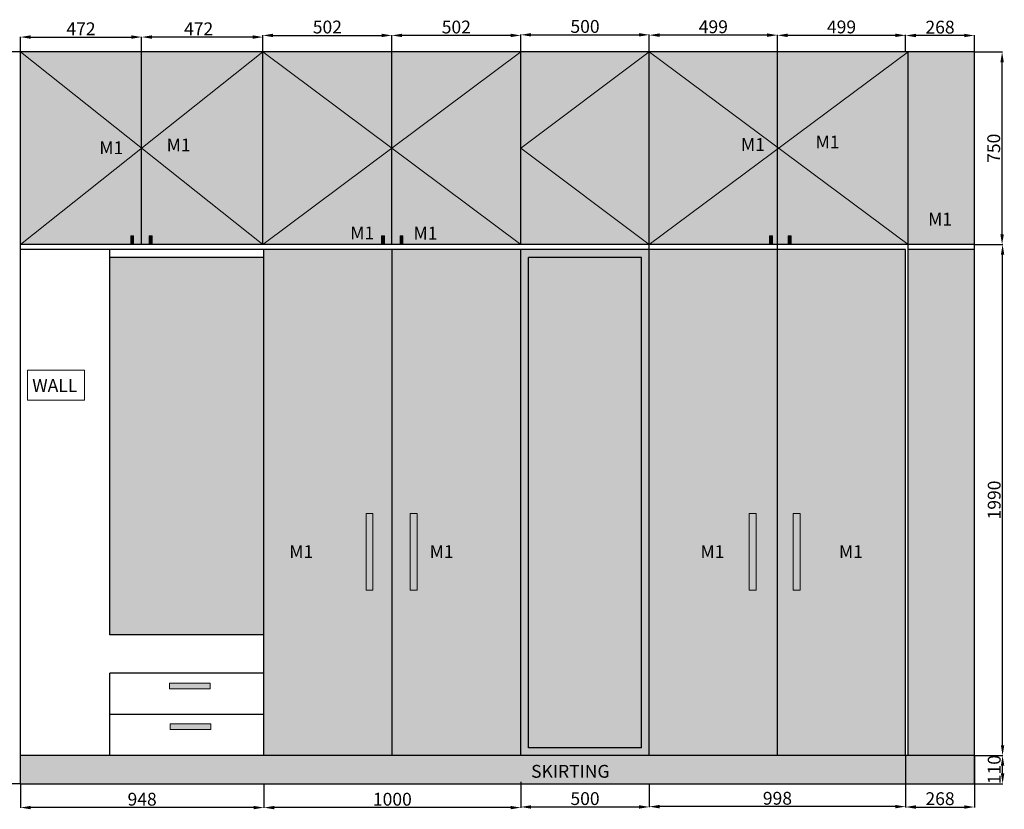
# Model space of a CAD drawing. Units: millimetres. Extents: x 46070 to 59439, y 6883 to 14761.
# Tile 2 of 5: x 49997 to 53830, y 6883 to 9959. Entities that reach past the tile are written whole.
import ezdxf

# ---------------------------------------------------------------- set-up
doc = ezdxf.new("R2010")
doc.units = ezdxf.units.MM
for name, color, linetype, lineweight in [('A-ANNO-DIMS', 2, 'Continuous', 18), ('A-ANNO-TEXT', 7, 'Continuous', 18), ('A-ELEV', 7, 'Continuous', 25), ('A-ELEV-OPEN', 1, 'Continuous', 13), ('A-ELEV-PATT', 8, 'Continuous', 13), ('A-FURN-HDWR', 4, 'Continuous', 18)]:
    doc.layers.add(name, color=color, linetype=linetype, lineweight=lineweight)
doc.styles.get("Standard").update_dxf_attribs({"font": 'arial.ttf'})
doc.dimstyles.new('ISO-25', dxfattribs={"dimtxt": 50, "dimasz": 40, "dimexe": 1.25, "dimexo": 0.625, "dimtad": 1, "dimtxsty": 'Standard', "dimcen": 2.5, "dimadec": 0, "dimazin": 0, "dimtfac": 1, "dimtmove": 0, "dimatfit": 3, "dimfxl": 1, "dimarcsym": 0})

# ---------------------------------------------------------------- blocks, each defined once
blk = doc.blocks.new('*D88')
at = {"layer": 'A-ANNO-DIMS', "color": 0, "lineweight": -2, "transparency": 16777216}
for p, q in [((53714.7, 7093.2), (53824.9, 7093.2)), ((53823.6, 7023.2), (53823.6, 7053.2)), ((53714.7, 6983.2), (53824.9, 6983.2))]:
    blk.add_line(p, q, dxfattribs=at)
at = {"layer": 'A-ANNO-DIMS', "color": 0, "transparency": 16777216}
for points in [[(53817, 7053.2), (53830.3, 7053.2), (53823.6, 7093.2)], [(53817, 7023.2), (53830.3, 7023.2), (53823.6, 6983.2)]]:
    blk.add_solid(points, dxfattribs=at)
at = {"layer": 'Defpoints', "color": 0, "transparency": 16777216}
for p in [(53714.1, 7093.2), (53823.6, 7093.2), (53714.1, 6983.2)]:
    blk.add_point(p, dxfattribs=at)
at = {"layer": 'A-ANNO-DIMS', "color": 0, "transparency": 16777216, "insert": (53797.5, 7038.1), "char_height": 50, "attachment_point": 5, "rotation": 90}
blk.add_mtext('110', dxfattribs=at)
blk = doc.blocks.new('*D80')
at = {"layer": 'A-ANNO-DIMS', "color": 0, "lineweight": -2, "transparency": 16777216}
for p, q in [((53714.7, 9083.2), (53824.8, 9083.2)), ((53823.5, 7133.2), (53823.5, 9043.2)), ((53714.7, 7093.2), (53824.8, 7093.2))]:
    blk.add_line(p, q, dxfattribs=at)
at = {"layer": 'A-ANNO-DIMS', "color": 0, "transparency": 16777216}
for points in [[(53816.8, 9043.2), (53830.2, 9043.2), (53823.5, 9083.2)], [(53816.8, 7133.2), (53830.2, 7133.2), (53823.5, 7093.2)]]:
    blk.add_solid(points, dxfattribs=at)
at = {"layer": 'Defpoints', "color": 0, "transparency": 16777216}
for p in [(53714.1, 9083.2), (53823.5, 9083.2), (53714.1, 7093.2)]:
    blk.add_point(p, dxfattribs=at)
at = {"layer": 'A-ANNO-DIMS', "color": 0, "transparency": 16777216, "insert": (53797.4, 8088.2), "char_height": 50, "attachment_point": 5, "rotation": 90}
blk.add_mtext('1990', dxfattribs=at)
blk = doc.blocks.new('*D89')
at = {"layer": 'A-ANNO-DIMS', "color": 0, "lineweight": -2, "transparency": 16777216}
for p, q in [((53714.7, 9833.2), (53823, 9833.2)), ((53821.7, 9123.2), (53821.7, 9793.2)), ((53714.7, 9083.2), (53823, 9083.2))]:
    blk.add_line(p, q, dxfattribs=at)
at = {"layer": 'A-ANNO-DIMS', "color": 0, "transparency": 16777216}
for points in [[(53815.1, 9793.2), (53828.4, 9793.2), (53821.7, 9833.2)], [(53815.1, 9123.2), (53828.4, 9123.2), (53821.7, 9083.2)]]:
    blk.add_solid(points, dxfattribs=at)
at = {"layer": 'Defpoints', "color": 0, "transparency": 16777216}
for p in [(53714.1, 9833.2), (53821.7, 9833.2), (53714.1, 9083.2)]:
    blk.add_point(p, dxfattribs=at)
at = {"layer": 'A-ANNO-DIMS', "color": 0, "transparency": 16777216, "insert": (53795.6, 9458.2), "char_height": 50, "attachment_point": 5, "rotation": 90}
blk.add_mtext('750', dxfattribs=at)
blk = doc.blocks.new('*D81')
at = {"layer": 'A-ANNO-DIMS', "color": 0, "lineweight": -2, "transparency": 16777216}
for p, q in [((52448.1, 9833.9), (52448.1, 9900)), ((52907.1, 9898.8), (52488.1, 9898.8)), ((52947.1, 9833.9), (52947.1, 9900))]:
    blk.add_line(p, q, dxfattribs=at)
at = {"layer": 'A-ANNO-DIMS', "color": 0, "transparency": 16777216}
for points in [[(52488.1, 9905.5), (52488.1, 9892.1), (52448.1, 9898.8)], [(52907.1, 9905.5), (52907.1, 9892.1), (52947.1, 9898.8)]]:
    blk.add_solid(points, dxfattribs=at)
at = {"layer": 'Defpoints', "color": 0, "transparency": 16777216}
for p in [(52448.1, 9898.8), (52448.1, 9833.2), (52947.1, 9833.2)]:
    blk.add_point(p, dxfattribs=at)
at = {"layer": 'A-ANNO-DIMS', "color": 0, "transparency": 16777216, "insert": (52697.6, 9925), "char_height": 50, "attachment_point": 5}
blk.add_mtext('499', dxfattribs=at)
blk = doc.blocks.new('*D82')
at = {"layer": 'A-ANNO-DIMS', "color": 0, "lineweight": -2, "transparency": 16777216}
for p, q in [((52947.1, 9833.9), (52947.1, 9899.4)), ((52987.1, 9898.1), (53406.1, 9898.1)), ((53446.1, 9833.9), (53446.1, 9899.4))]:
    blk.add_line(p, q, dxfattribs=at)
at = {"layer": 'A-ANNO-DIMS', "color": 0, "transparency": 16777216}
for points in [[(52987.1, 9904.8), (52987.1, 9891.4), (52947.1, 9898.1)], [(53406.1, 9904.8), (53406.1, 9891.4), (53446.1, 9898.1)]]:
    blk.add_solid(points, dxfattribs=at)
at = {"layer": 'Defpoints', "color": 0, "transparency": 16777216}
for p in [(53446.1, 9898.1), (52947.1, 9833.2), (53446.1, 9833.2)]:
    blk.add_point(p, dxfattribs=at)
at = {"layer": 'A-ANNO-DIMS', "color": 0, "transparency": 16777216, "insert": (53196.6, 9924.3), "char_height": 50, "attachment_point": 5}
blk.add_mtext('499', dxfattribs=at)
blk = doc.blocks.new('*D83')
at = {"layer": 'A-ANNO-DIMS', "color": 0, "lineweight": -2, "transparency": 16777216}
for p, q in [((52448.1, 6982.6), (52448.1, 6892.6)), ((53446.1, 6982.6), (53446.1, 6892.6)), ((53406.1, 6893.8), (52488.1, 6893.8))]:
    blk.add_line(p, q, dxfattribs=at)
at = {"layer": 'A-ANNO-DIMS', "color": 0, "transparency": 16777216}
for points in [[(52488.1, 6900.5), (52488.1, 6887.2), (52448.1, 6893.8)], [(53406.1, 6900.5), (53406.1, 6887.2), (53446.1, 6893.8)]]:
    blk.add_solid(points, dxfattribs=at)
at = {"layer": 'Defpoints', "color": 0, "transparency": 16777216}
for p in [(52448.1, 6983.2), (53446.1, 6983.2), (52448.1, 6893.8)]:
    blk.add_point(p, dxfattribs=at)
at = {"layer": 'A-ANNO-DIMS', "color": 0, "transparency": 16777216, "insert": (52947.1, 6920), "char_height": 50, "attachment_point": 5}
blk.add_mtext('998', dxfattribs=at)
blk = doc.blocks.new('*D84')
at = {"layer": 'A-ANNO-DIMS', "color": 0, "lineweight": -2, "transparency": 16777216}
for p, q in [((51948.1, 6982.6), (51948.1, 6891.3)), ((52448.1, 6982.6), (52448.1, 6891.3)), ((51988.1, 6892.6), (52408.1, 6892.6))]:
    blk.add_line(p, q, dxfattribs=at)
at = {"layer": 'A-ANNO-DIMS', "color": 0, "transparency": 16777216}
for points in [[(51988.1, 6899.3), (51988.1, 6885.9), (51948.1, 6892.6)], [(52408.1, 6899.3), (52408.1, 6885.9), (52448.1, 6892.6)]]:
    blk.add_solid(points, dxfattribs=at)
at = {"layer": 'Defpoints', "color": 0, "transparency": 16777216}
for p in [(51948.1, 6983.2), (52448.1, 6983.2), (52448.1, 6892.6)]:
    blk.add_point(p, dxfattribs=at)
at = {"layer": 'A-ANNO-DIMS', "color": 0, "transparency": 16777216, "insert": (52198.1, 6918.7), "char_height": 50, "attachment_point": 5}
blk.add_mtext('500', dxfattribs=at)
blk = doc.blocks.new('*D93')
at = {"layer": 'A-ANNO-DIMS', "color": 0, "lineweight": -2, "transparency": 16777216}
for p, q in [((51948.1, 9833.9), (51948.1, 9901.3)), ((51988.1, 9900), (52408.1, 9900)), ((52448.1, 9833.9), (52448.1, 9901.3))]:
    blk.add_line(p, q, dxfattribs=at)
at = {"layer": 'A-ANNO-DIMS', "color": 0, "transparency": 16777216}
for points in [[(51988.1, 9906.7), (51988.1, 9893.4), (51948.1, 9900)], [(52408.1, 9906.7), (52408.1, 9893.4), (52448.1, 9900)]]:
    blk.add_solid(points, dxfattribs=at)
at = {"layer": 'Defpoints', "color": 0, "transparency": 16777216}
for p in [(52448.1, 9900), (51948.1, 9833.2), (52448.1, 9833.2)]:
    blk.add_point(p, dxfattribs=at)
at = {"layer": 'A-ANNO-DIMS', "color": 0, "transparency": 16777216, "insert": (52198.1, 9926.2), "char_height": 50, "attachment_point": 5}
blk.add_mtext('500', dxfattribs=at)
blk = doc.blocks.new('*D90')
at = {"layer": 'A-ANNO-DIMS', "color": 0, "lineweight": -2, "transparency": 16777216}
for p, q in [((51446.1, 9833.9), (51446.1, 9899)), ((51908.1, 9897.7), (51486.1, 9897.7)), ((51948.1, 9833.9), (51948.1, 9899))]:
    blk.add_line(p, q, dxfattribs=at)
at = {"layer": 'A-ANNO-DIMS', "color": 0, "transparency": 16777216}
for points in [[(51486.1, 9904.4), (51486.1, 9891.1), (51446.1, 9897.7)], [(51908.1, 9904.4), (51908.1, 9891.1), (51948.1, 9897.7)]]:
    blk.add_solid(points, dxfattribs=at)
at = {"layer": 'Defpoints', "color": 0, "transparency": 16777216}
for p in [(51446.1, 9897.7), (51446.1, 9833.2), (51948.1, 9833.2)]:
    blk.add_point(p, dxfattribs=at)
at = {"layer": 'A-ANNO-DIMS', "color": 0, "transparency": 16777216, "insert": (51697.1, 9923.9), "char_height": 50, "attachment_point": 5}
blk.add_mtext('502', dxfattribs=at)
blk = doc.blocks.new('*D91')
at = {"layer": 'A-ANNO-DIMS', "color": 0, "lineweight": -2, "transparency": 16777216}
for p, q in [((50472.1, 9833.9), (50472.1, 9892.5)), ((50904.1, 9891.3), (50512.1, 9891.3)), ((50944.1, 9833.9), (50944.1, 9892.5))]:
    blk.add_line(p, q, dxfattribs=at)
at = {"layer": 'A-ANNO-DIMS', "color": 0, "transparency": 16777216}
for points in [[(50512.1, 9898), (50512.1, 9884.6), (50472.1, 9891.3)], [(50904.1, 9898), (50904.1, 9884.6), (50944.1, 9891.3)]]:
    blk.add_solid(points, dxfattribs=at)
at = {"layer": 'Defpoints', "color": 0, "transparency": 16777216}
for p in [(50472.1, 9891.3), (50472.1, 9833.2), (50944.1, 9833.2)]:
    blk.add_point(p, dxfattribs=at)
at = {"layer": 'A-ANNO-DIMS', "color": 0, "transparency": 16777216, "insert": (50694, 9917), "char_height": 50, "attachment_point": 5}
blk.add_mtext('472', dxfattribs=at)
blk = doc.blocks.new('*D85')
at = {"layer": 'A-ANNO-DIMS', "color": 0, "lineweight": -2, "transparency": 16777216}
for p, q in [((50944.1, 9833.9), (50944.1, 9899)), ((50984.1, 9897.7), (51406.1, 9897.7)), ((51446.1, 9833.9), (51446.1, 9899))]:
    blk.add_line(p, q, dxfattribs=at)
at = {"layer": 'A-ANNO-DIMS', "color": 0, "transparency": 16777216}
for points in [[(50984.1, 9904.4), (50984.1, 9891.1), (50944.1, 9897.7)], [(51406.1, 9904.4), (51406.1, 9891.1), (51446.1, 9897.7)]]:
    blk.add_solid(points, dxfattribs=at)
at = {"layer": 'Defpoints', "color": 0, "transparency": 16777216}
for p in [(51446.1, 9897.7), (50944.1, 9833.2), (51446.1, 9833.2)]:
    blk.add_point(p, dxfattribs=at)
at = {"layer": 'A-ANNO-DIMS', "color": 0, "transparency": 16777216, "insert": (51195.1, 9923.9), "char_height": 50, "attachment_point": 5}
blk.add_mtext('502', dxfattribs=at)
blk = doc.blocks.new('*D92')
at = {"layer": 'A-ANNO-DIMS', "color": 0, "lineweight": -2, "transparency": 16777216}
for p, q in [((50000.1, 9833.9), (50000.1, 9892.6)), ((50040.1, 9891.3), (50432.1, 9891.3)), ((50472.1, 9833.9), (50472.1, 9892.6))]:
    blk.add_line(p, q, dxfattribs=at)
at = {"layer": 'A-ANNO-DIMS', "color": 0, "transparency": 16777216}
for points in [[(50040.1, 9898), (50040.1, 9884.7), (50000.1, 9891.3)], [(50432.1, 9898), (50432.1, 9884.7), (50472.1, 9891.3)]]:
    blk.add_solid(points, dxfattribs=at)
at = {"layer": 'Defpoints', "color": 0, "transparency": 16777216}
for p in [(50472.1, 9891.3), (50000.1, 9833.2), (50472.1, 9833.2)]:
    blk.add_point(p, dxfattribs=at)
at = {"layer": 'A-ANNO-DIMS', "color": 0, "transparency": 16777216, "insert": (50236.1, 9917.1), "char_height": 50, "attachment_point": 5}
blk.add_mtext('472', dxfattribs=at)
blk = doc.blocks.new('*D94')
at = {"layer": 'A-ANNO-DIMS', "color": 0, "lineweight": -2, "transparency": 16777216}
for p, q in [((53446.1, 9833.9), (53446.1, 9898.6)), ((53674.1, 9897.4), (53486.1, 9897.4)), ((53714.1, 9833.9), (53714.1, 9898.6))]:
    blk.add_line(p, q, dxfattribs=at)
at = {"layer": 'A-ANNO-DIMS', "color": 0, "transparency": 16777216}
for points in [[(53486.1, 9904.1), (53486.1, 9890.7), (53446.1, 9897.4)], [(53674.1, 9904.1), (53674.1, 9890.7), (53714.1, 9897.4)]]:
    blk.add_solid(points, dxfattribs=at)
at = {"layer": 'Defpoints', "color": 0, "transparency": 16777216}
for p in [(53446.1, 9897.4), (53446.1, 9833.2), (53714.1, 9833.2)]:
    blk.add_point(p, dxfattribs=at)
at = {"layer": 'A-ANNO-DIMS', "color": 0, "transparency": 16777216, "insert": (53580.1, 9923.5), "char_height": 50, "attachment_point": 5}
blk.add_mtext('268', dxfattribs=at)
blk = doc.blocks.new('*D86')
at = {"layer": 'A-ANNO-DIMS', "color": 0, "lineweight": -2, "transparency": 16777216}
for p, q in [((50948.1, 6982.6), (50948.1, 6888.8)), ((51948.1, 6990.1), (51948.1, 6888.8)), ((51908.1, 6890.1), (50988.1, 6890.1))]:
    blk.add_line(p, q, dxfattribs=at)
at = {"layer": 'A-ANNO-DIMS', "color": 0, "transparency": 16777216}
for points in [[(50988.1, 6896.7), (50988.1, 6883.4), (50948.1, 6890.1)], [(51908.1, 6896.7), (51908.1, 6883.4), (51948.1, 6890.1)]]:
    blk.add_solid(points, dxfattribs=at)
at = {"layer": 'Defpoints', "color": 0, "transparency": 16777216}
for p in [(50948.1, 6983.2), (51948.1, 6990.7), (50948.1, 6890.1)]:
    blk.add_point(p, dxfattribs=at)
at = {"layer": 'A-ANNO-DIMS', "color": 0, "transparency": 16777216, "insert": (51448.1, 6916.2), "char_height": 50, "attachment_point": 5}
blk.add_mtext('1000', dxfattribs=at)
blk = doc.blocks.new('*D87')
at = {"layer": 'A-ANNO-DIMS', "color": 0, "lineweight": -2, "transparency": 16777216}
for p, q in [((50000.1, 6982.6), (50000.1, 6888.9)), ((50948.1, 6982.6), (50948.1, 6888.9)), ((50908.1, 6890.2), (50040.1, 6890.2))]:
    blk.add_line(p, q, dxfattribs=at)
at = {"layer": 'A-ANNO-DIMS', "color": 0, "transparency": 16777216}
for points in [[(50040.1, 6896.8), (50040.1, 6883.5), (50000.1, 6890.2)], [(50908.1, 6896.8), (50908.1, 6883.5), (50948.1, 6890.2)]]:
    blk.add_solid(points, dxfattribs=at)
at = {"layer": 'Defpoints', "color": 0, "transparency": 16777216}
for p in [(50000.1, 6983.2), (50948.1, 6983.2), (50000.1, 6890.2)]:
    blk.add_point(p, dxfattribs=at)
at = {"layer": 'A-ANNO-DIMS', "color": 0, "transparency": 16777216, "insert": (50474.1, 6916.3), "char_height": 50, "attachment_point": 5}
blk.add_mtext('948', dxfattribs=at)
blk = doc.blocks.new('*D95')
at = {"layer": 'A-ANNO-DIMS', "color": 0, "lineweight": -2, "transparency": 16777216}
for p, q in [((53446.1, 7092.6), (53446.1, 6891)), ((53714.1, 7092.6), (53714.1, 6891)), ((53486.1, 6892.3), (53674.1, 6892.3))]:
    blk.add_line(p, q, dxfattribs=at)
at = {"layer": 'A-ANNO-DIMS', "color": 0, "transparency": 16777216}
for points in [[(53486.1, 6899), (53486.1, 6885.6), (53446.1, 6892.3)], [(53674.1, 6899), (53674.1, 6885.6), (53714.1, 6892.3)]]:
    blk.add_solid(points, dxfattribs=at)
at = {"layer": 'Defpoints', "color": 0, "transparency": 16777216}
for p in [(53446.1, 7093.2), (53714.1, 7093.2), (53714.1, 6892.3)]:
    blk.add_point(p, dxfattribs=at)
at = {"layer": 'A-ANNO-DIMS', "color": 0, "transparency": 16777216, "insert": (53580.1, 6918.4), "char_height": 50, "attachment_point": 5}
blk.add_mtext('268', dxfattribs=at)
blk = doc.blocks.new('*D96')
at = {"layer": 'A-ANNO-DIMS', "color": 0, "lineweight": -2, "transparency": 16777216}
for p, q in [((49999.5, 9833.2), (49847.1, 9833.2)), ((49848.4, 7023.2), (49848.4, 9793.2)), ((49999.5, 6983.2), (49847.1, 6983.2))]:
    blk.add_line(p, q, dxfattribs=at)
at = {"layer": 'A-ANNO-DIMS', "color": 0, "transparency": 16777216}
for points in [[(49841.7, 9793.2), (49855, 9793.2), (49848.4, 9833.2)], [(49841.7, 7023.2), (49855, 7023.2), (49848.4, 6983.2)]]:
    blk.add_solid(points, dxfattribs=at)
at = {"layer": 'Defpoints', "color": 0, "transparency": 16777216}
for p in [(49848.4, 9833.2), (50000.1, 9833.2), (50000.1, 6983.2)]:
    blk.add_point(p, dxfattribs=at)
at = {"layer": 'A-ANNO-DIMS', "color": 0, "transparency": 16777216, "insert": (49822.2, 8408.2), "char_height": 50, "attachment_point": 5, "rotation": 90}
blk.add_mtext('2850', dxfattribs=at)
blk = doc.blocks.new('HANDLE-BAR-300')
blk.add_lwpolyline([(0, 299.3), (26.9, 299.3), (26.9, 0), (0, 0)], close=True)
blk = doc.blocks.new('DRAWER-PULL-160')
blk.add_lwpolyline([(0, 22.3), (158.3, 22.3), (158.3, 0), (0, 0)], close=True)
blk = doc.blocks.new('LOFT-KNOB')
blk.add_lwpolyline([(0, 33.9), (11, 33.9), (11, 0), (0, 0)], close=True)

msp = doc.modelspace()

# ---------------------------------------------------------------- hatches: boundary and pattern name
at = {"layer": 'A-ELEV-PATT'}
h = msp.add_hatch(color=256, dxfattribs=at)
h.dxf.hatch_style = 1
h.paths.add_polyline_path([(53714.11, 7093.249), (50000.11, 7093.249), (50000.11, 6983.249), (53714.11, 6983.249)])
h.paths.add_polyline_path([(50472.11, 9833.249), (50000.11, 9833.249), (50472.11, 9458.249)], flags=17)
h.paths.add_polyline_path([(50944.11, 9833.249), (50472.11, 9833.249), (50472.11, 9458.249)], flags=17)
h.paths.add_polyline_path([(50944.11, 9833.249), (50472.11, 9458.249), (50944.11, 9083.249)])
h.paths.add_polyline_path([(50472.11, 9458.249), (50472.11, 9083.249), (50502.002, 9083.249), (50502.002, 9117.126), (50512.998, 9117.126), (50512.998, 9083.249), (50944.11, 9083.249)])
h.paths.add_polyline_path([(50472.11, 9458.249), (50000.11, 9083.249), (50429.849, 9083.249), (50429.849, 9117.126), (50440.845, 9117.126), (50440.845, 9083.249), (50472.11, 9083.249)])
h.paths.add_polyline_path([(50000.11, 9833.249), (50000.11, 9083.249), (50472.11, 9458.249)])
h.paths.add_polyline_path([(50944.11, 9833.249), (50944.11, 9083.249), (51446.11, 9458.249)])
h.paths.add_polyline_path([(51446.11, 9833.249), (50944.11, 9833.249), (51446.11, 9458.249)])
h.paths.add_polyline_path([(51948.11, 9833.249), (51446.11, 9833.249), (51446.11, 9458.249)], flags=17)
h.paths.add_polyline_path([(51948.11, 9833.249), (51446.11, 9458.249), (51948.11, 9083.249)])
h.paths.add_polyline_path([(51446.11, 9458.249), (51446.11, 9083.249), (51478.071, 9083.249), (51478.071, 9117.126), (51489.067, 9117.126), (51489.067, 9083.249), (51948.11, 9083.249)], flags=17)
h.paths.add_polyline_path([(51446.11, 9458.249), (50944.11, 9083.249), (51405.918, 9083.249), (51405.918, 9117.126), (51416.914, 9117.126), (51416.914, 9083.249), (51446.11, 9083.249)], flags=17)
h.paths.add_polyline_path([(52448.11, 9833.249), (51948.11, 9458.249), (52448.11, 9083.249)])
h.paths.add_polyline_path([(52448.11, 9833.249), (51948.11, 9833.249), (51948.11, 9458.249)])
h.paths.add_polyline_path([(51948.11, 9458.249), (51948.11, 9083.249), (52448.11, 9083.249)])
h.paths.add_polyline_path([(52947.11, 9454.529), (52947.11, 9461.969), (52448.11, 9833.249), (52448.11, 9083.249)])
h.paths.add_polyline_path([(52947.11, 9833.249), (52448.11, 9833.249), (52947.11, 9461.969)])
h.paths.add_polyline_path([(52947.11, 9454.529), (52448.11, 9083.249), (52916.868, 9083.249), (52916.868, 9117.126), (52927.864, 9117.126), (52927.864, 9083.249), (52947.11, 9083.249)], flags=17)
h.paths.add_polyline_path([(52952.11, 9458.249), (52947.11, 9454.529), (52947.11, 9083.249), (52989.021, 9083.249), (52989.021, 9117.126), (53000.017, 9117.126), (53000.017, 9083.249), (53456.11, 9083.249)])
h.paths.add_polyline_path([(53456.11, 9833.249), (52952.11, 9458.249), (53456.11, 9083.249)])
h.paths.add_polyline_path([(53456.11, 9833.249), (52947.11, 9833.249), (52947.11, 9461.969), (52952.11, 9458.249)])
h.paths.add_polyline_path([(53714.11, 9833.249), (53456.11, 9833.249), (53456.11, 9083.249), (53714.11, 9083.249)])
h.paths.add_polyline_path([(51972.606, 6978.221), (52327.483, 6978.221), (52327.483, 7081.256), (51972.606, 7081.256)], flags=9)
h.paths.add_polyline_path([(50551.779, 9418.51), (50673.812, 9418.51), (50673.812, 9521.545), (50551.779, 9521.545)], flags=24)
h.paths.add_polyline_path([(50289.669, 9407.696), (50411.702, 9407.696), (50411.702, 9510.731), (50289.669, 9510.731)], flags=24)
h.paths.add_polyline_path([(51512.708, 9075.067), (51634.741, 9075.067), (51634.741, 9178.103), (51512.708, 9178.103)], flags=9)
h.paths.add_polyline_path([(51266.468, 9075.686), (51388.5, 9075.686), (51388.5, 9178.722), (51266.468, 9178.722)], flags=9)
h.paths.add_polyline_path([(52787.384, 9420.123), (52909.417, 9420.123), (52909.417, 9523.158), (52787.384, 9523.158)], flags=24)
h.paths.add_polyline_path([(53077.89, 9429.964), (53199.923, 9429.964), (53199.923, 9533), (53077.89, 9533)], flags=24)
h.paths.add_polyline_path([(53516.108, 9129.796), (53638.141, 9129.796), (53638.141, 9232.831), (53516.108, 9232.831)], flags=24)
h = msp.add_hatch(color=256, dxfattribs=at)
h.dxf.hatch_style = 1
h.paths.add_polyline_path([(50429.849, 9083.249), (50440.845, 9083.249), (50440.845, 9117.126), (50429.849, 9117.126)])
h = msp.add_hatch(color=256, dxfattribs=at)
h.dxf.hatch_style = 1
h.paths.add_polyline_path([(50502.002, 9083.249), (50512.998, 9083.249), (50512.998, 9117.126), (50502.002, 9117.126)])
h = msp.add_hatch(color=256, dxfattribs=at)
h.dxf.hatch_style = 1
h.paths.add_polyline_path([(51416.914, 9117.126), (51405.918, 9117.126), (51405.918, 9083.249), (51416.914, 9083.249)])
h = msp.add_hatch(color=256, dxfattribs=at)
h.dxf.hatch_style = 1
h.paths.add_polyline_path([(51489.067, 9117.126), (51478.071, 9117.126), (51478.071, 9083.249), (51489.067, 9083.249)])
h = msp.add_hatch(color=256, dxfattribs=at)
h.dxf.hatch_style = 1
h.paths.add_polyline_path([(52927.864, 9117.126), (52916.868, 9117.126), (52916.868, 9083.249), (52927.864, 9083.249)])
h = msp.add_hatch(color=256, dxfattribs=at)
h.dxf.hatch_style = 1
h.paths.add_polyline_path([(53000.017, 9117.126), (52989.021, 9117.126), (52989.021, 9083.249), (53000.017, 9083.249)])
h = msp.add_hatch(color=256, dxfattribs=at)
h.dxf.hatch_style = 1
h.paths.add_polyline_path([(51446.11, 7093.249), (51948.11, 7093.249), (51948.11, 9063.249), (51446.11, 9063.249)])
h.paths.add_polyline_path([(51544.488, 7736.671), (51517.57, 7736.671), (51517.57, 8035.954), (51544.488, 8035.954)], flags=16)
h.paths.add_polyline_path([(51446.11, 9063.249), (50948.11, 9063.249), (50948.11, 7093.249), (51446.11, 7093.249)])
h.paths.add_polyline_path([(51345.742, 7736.671), (51345.742, 8035.954), (51372.66, 8035.954), (51372.66, 7736.671)], flags=16)
h.paths.add_polyline_path([(51575.599, 7834.506), (51697.632, 7834.506), (51697.632, 7937.541), (51575.599, 7937.541)], flags=24)
h.paths.add_polyline_path([(51029.15, 7834.506), (51151.183, 7834.506), (51151.183, 7937.541), (51029.15, 7937.541)], flags=24)
h = msp.add_hatch(color=256, dxfattribs=at)
h.dxf.hatch_style = 1
h.paths.add_polyline_path([(52448.11, 9063.249), (51948.11, 9063.249), (51948.11, 7093.249), (52448.11, 7093.249)])
h.paths.add_polyline_path([(52418.11, 7123.249), (51978.11, 7123.249), (51978.11, 9033.249), (52418.11, 9033.249)], flags=16)
h = msp.add_hatch(color=256, dxfattribs=at)
h.dxf.hatch_style = 1
h.paths.add_polyline_path([(52947.11, 9063.249), (52448.11, 9063.249), (52448.11, 7093.249), (52947.11, 7093.249)])
h.paths.add_polyline_path([(52836.849, 7736.671), (52836.849, 8035.954), (52863.767, 8035.954), (52863.767, 7736.671)], flags=16)
h.paths.add_polyline_path([(52947.11, 7093.249), (53446.11, 7093.249), (53446.11, 9063.249), (52947.11, 9063.249)])
h.paths.add_polyline_path([(53035.595, 7736.671), (53008.677, 7736.671), (53008.677, 8035.954), (53035.595, 8035.954)], flags=16)
h.paths.add_polyline_path([(52629.716, 7834.506), (52751.749, 7834.506), (52751.749, 7937.541), (52629.716, 7937.541)], flags=24)
h.paths.add_polyline_path([(53168.926, 7834.506), (53290.959, 7834.506), (53290.959, 7937.541), (53168.926, 7937.541)], flags=24)
h = msp.add_hatch(color=256, dxfattribs=at)
h.dxf.hatch_style = 1
h.paths.add_polyline_path([(53456.11, 7093.249), (53714.11, 7093.249), (53714.11, 9063.249), (53456.11, 9063.249)])
h = msp.add_hatch(color=256, dxfattribs=at)
h.dxf.hatch_style = 1
h.paths.add_polyline_path([(50948.11, 9033.249), (50348.11, 9033.249), (50348.11, 7563.249), (50948.11, 7563.249)])
h = msp.add_hatch(color=256, dxfattribs=at)
h.dxf.hatch_style = 1
h.paths.add_polyline_path([(52418.11, 9033.249), (51978.11, 9033.249), (51978.11, 7123.249), (52418.11, 7123.249)])
h = msp.add_hatch(color=256, dxfattribs=at)
h.dxf.hatch_style = 1
h.paths.add_polyline_path([(51517.57, 7736.671), (51544.488, 7736.671), (51544.488, 8035.954), (51517.57, 8035.954)])
h.paths.add_polyline_path([(51345.742, 7736.671), (51372.66, 7736.671), (51372.66, 8035.954), (51345.742, 8035.954)])
h = msp.add_hatch(color=256, dxfattribs=at)
h.dxf.hatch_style = 1
h.paths.add_polyline_path([(53008.677, 7736.671), (53035.595, 7736.671), (53035.595, 8035.954), (53008.677, 8035.954)])
h.paths.add_polyline_path([(52836.849, 7736.671), (52863.767, 7736.671), (52863.767, 8035.954), (52836.849, 8035.954)])
h = msp.add_hatch(color=256, dxfattribs=at)
h.dxf.hatch_style = 1
h.paths.add_polyline_path([(50580.903, 7375.11), (50580.903, 7352.845), (50739.206, 7352.845), (50739.206, 7375.11)])
h.paths.add_polyline_path([(50741.55, 7194.642), (50741.55, 7216.907), (50583.248, 7216.907), (50583.248, 7194.642)])

# ---------------------------------------------------------------- linework, layer by layer
at = {"layer": 'A-ANNO-TEXT'}
msp.add_lwpolyline([(50027.231, 8594.172), (50249.138, 8594.172), (50249.138, 8477.325), (50027.231, 8477.325)], close=True, dxfattribs=at)
at = {"layer": 'A-ELEV'}
for p, q in [((50000.11, 6983.249), (50000.11, 9833.249)), ((53714.11, 9833.249), (50000.11, 9833.249)), ((50472.11, 9083.249), (50472.11, 9833.249)), ((50944.11, 9083.249), (50944.11, 9833.249)), ((51446.11, 9083.249), (51446.11, 9833.249)), ((51948.11, 9083.249), (51948.11, 9833.249)), ((52448.11, 7093.249), (52448.11, 9833.249)), ((52947.11, 9063.249), (52947.11, 9833.249)), ((53456.11, 7093.249), (53456.11, 9833.249)), ((53714.11, 6983.249), (53714.11, 9833.249)), ((53714.11, 9083.249), (50000.11, 9083.249)), ((53446.11, 9063.249), (50000.11, 9063.249)), ((50348.11, 7563.249), (50348.11, 9063.249)), ((50948.11, 7093.249), (50948.11, 9063.249)), ((51446.11, 9063.249), (51446.11, 7093.249)), ((51948.11, 7093.249), (51948.11, 9063.249)), ((52947.11, 7093.249), (52947.11, 9063.249)), ((53446.11, 7093.249), (53446.11, 9063.249)), ((53714.11, 9063.249), (53456.11, 9063.249)), ((50948.11, 9033.249), (50348.11, 9033.249)), ((51978.11, 7123.249), (51978.11, 9033.249)), ((52418.11, 9033.249), (51978.11, 9033.249)), ((52418.11, 7123.249), (52418.11, 9033.249)), ((50948.11, 7563.249), (50348.11, 7563.249)), ((50348.11, 7093.249), (50348.11, 7413.249)), ((50948.11, 7413.249), (50348.11, 7413.249)), ((50948.11, 7253.249), (50348.11, 7253.249)), ((53714.11, 7093.249), (50000.11, 7093.249)), ((52418.11, 7123.249), (51978.11, 7123.249)), ((50000.11, 6983.249), (53714.11, 6983.249))]:
    msp.add_line(p, q, dxfattribs=at)
at = {"layer": 'A-ELEV-OPEN'}
for p, q in [((50000.11, 9833.249), (50944.11, 9083.249)), ((50944.11, 9833.249), (50000.11, 9083.249)), ((50944.11, 9833.249), (51948.11, 9083.249)), ((51948.11, 9833.249), (50944.11, 9083.249)), ((52448.11, 9833.249), (51948.11, 9458.249)), ((52448.11, 9833.249), (53456.11, 9083.249)), ((52448.11, 9083.249), (53456.11, 9833.249)), ((51948.11, 9458.249), (52448.11, 9083.249))]:
    msp.add_line(p, q, dxfattribs=at)

# ---------------------------------------------------------------- block references
at = {"layer": 'A-FURN-HDWR'}
for name, p in [('LOFT-KNOB', (50429.849, 9083.249)), ('LOFT-KNOB', (50502.002, 9083.249)), ('LOFT-KNOB', (51405.918, 9083.249)), ('LOFT-KNOB', (51478.071, 9083.249)), ('LOFT-KNOB', (52916.868, 9083.249)), ('LOFT-KNOB', (52989.021, 9083.249)), ('HANDLE-BAR-300', (51345.742, 7736.671)), ('HANDLE-BAR-300', (51517.569, 7736.671)), ('HANDLE-BAR-300', (52836.849, 7736.671)), ('HANDLE-BAR-300', (53008.676, 7736.671)), ('DRAWER-PULL-160', (50580.904, 7352.845)), ('DRAWER-PULL-160', (50583.248, 7194.642))]:
    msp.add_blockref(name, p, dxfattribs=at)

# ---------------------------------------------------------------- texts
at = {"layer": 'A-ANNO-TEXT', "char_height": 50, "attachment_point": 1}
for s, insert in [('M1', (53095.574, 9507.471)), ('M1', (50307.353, 9485.203)), ('M1', (50569.464, 9496.017)), ('M1', (52805.068, 9497.63)), ('M1', (53533.792, 9207.302)), ('M1', (51284.152, 9153.193)), ('M1', (51530.393, 9152.574)), ('WALL', (50046.319, 8559.269)), ('M1', (51046.834, 7912.012)), ('M1', (51593.283, 7912.012)), ('M1', (52647.401, 7912.012)), ('M1', (53186.61, 7912.012)), ('SKIRTING ', (51988.244, 7056.376))]:
    msp.add_mtext_dynamic_manual_height_columns(s, width=502.17574, gutter_width=12.5, heights=[0], dxfattribs=dict(at, insert=insert))

# ---------------------------------------------------------------- dimensions: what is measured, and where the dimension line sits
at = {"layer": 'A-ANNO-DIMS'}
for base, p1, p2, picture, middle in [((50472.11, 9891.329), (50000.11, 9833.249), (50472.11, 9833.249), '*D92', (50236.11, 9917.056)), ((51446.11, 9897.72), (50944.11, 9833.249), (51446.11, 9833.249), '*D85', (51195.11, 9923.873)), ((51446.11, 9897.72), (51948.11, 9833.249), (51446.11, 9833.249), '*D90', (51697.11, 9923.873)), ((52448.11, 9900.048), (51948.11, 9833.249), (52448.11, 9833.249), '*D93', (52198.11, 9926.202)), ((52448.11, 9898.798), (52947.11, 9833.249), (52448.11, 9833.249), '*D81', (52697.61, 9924.952)), ((53446.11, 9898.105), (52947.11, 9833.249), (53446.11, 9833.249), '*D82', (53196.61, 9924.259)), ((53446.11, 9897.386), (53714.11, 9833.249), (53446.11, 9833.249), '*D94', (53580.11, 9923.54)), ((53714.11, 6892.288), (53446.11, 7093.249), (53714.11, 7093.249), '*D95', (53580.11, 6918.442)), ((50000.11, 6890.162), (50948.11, 6983.249), (50000.11, 6983.249), '*D87', (50474.11, 6916.316)), ((50948.11, 6890.072), (51948.11, 6990.723), (50948.11, 6983.249), '*D86', (51448.11, 6916.226)), ((52448.11, 6892.586), (51948.11, 6983.249), (52448.11, 6983.249), '*D84', (52198.11, 6918.74)), ((52448.11, 6893.836), (53446.11, 6983.249), (52448.11, 6983.249), '*D83', (52947.11, 6919.99))]:
    dim = msp.add_linear_dim(base=base, p1=p1, p2=p2, dimstyle='ISO-25', override={"dimclrd": 0, "dimclre": 0, "dimclrt": 0}, dxfattribs=at)
    dim.commit()
    dim.dimension.update_dxf_attribs({"geometry": picture, "text_midpoint": middle})
dim = msp.add_linear_dim(base=(50472.11, 9891.295), p1=(50944.11, 9833.249), p2=(50472.11, 9833.249), dimstyle='ISO-25', override={"dimclrd": 0, "dimclre": 0, "dimclrt": 0}, dxfattribs=at)
dim.commit()
dim.dimension.update_dxf_attribs({"geometry": '*D91', "text_midpoint": (50693.963, 9891.295), "dimtype": 160})
for base, p1, p2, picture, middle in [((49848.383, 9833.249), (50000.11, 6983.249), (50000.11, 9833.249), '*D96', (49822.229, 8408.249)), ((53821.726, 9833.249), (53714.11, 9083.249), (53714.11, 9833.249), '*D89', (53795.572, 9458.249))]:
    dim = msp.add_linear_dim(base=base, p1=p1, p2=p2, angle=90, dimstyle='ISO-25', override={"dimclrd": 0, "dimclre": 0, "dimclrt": 0}, dxfattribs=at)
    dim.commit()
    dim.dimension.update_dxf_attribs({"geometry": picture, "text_midpoint": middle})
for base, p1, p2, picture, middle in [((53823.504, 9083.249), (53714.11, 7093.249), (53714.11, 9083.249), '*D80', (53823.504, 8088.249)), ((53823.628, 7093.249), (53714.11, 6983.249), (53714.11, 7093.249), '*D88', (53823.628, 7038.147))]:
    dim = msp.add_linear_dim(base=base, p1=p1, p2=p2, angle=90, dimstyle='ISO-25', override={"dimclrd": 0, "dimclre": 0, "dimclrt": 0}, dxfattribs=at)
    dim.commit()
    dim.dimension.update_dxf_attribs({"geometry": picture, "text_midpoint": middle, "dimtype": 160})

doc.saveas('drawing.dxf')
